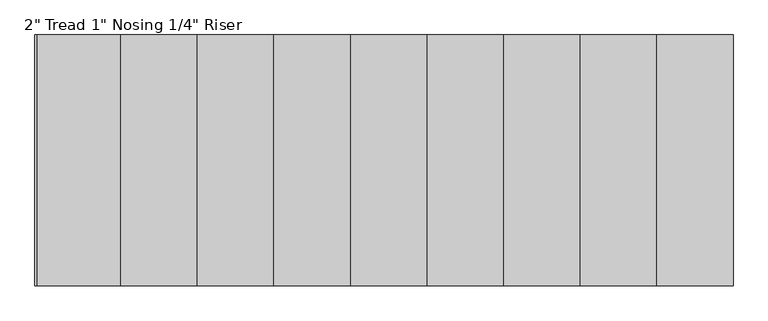
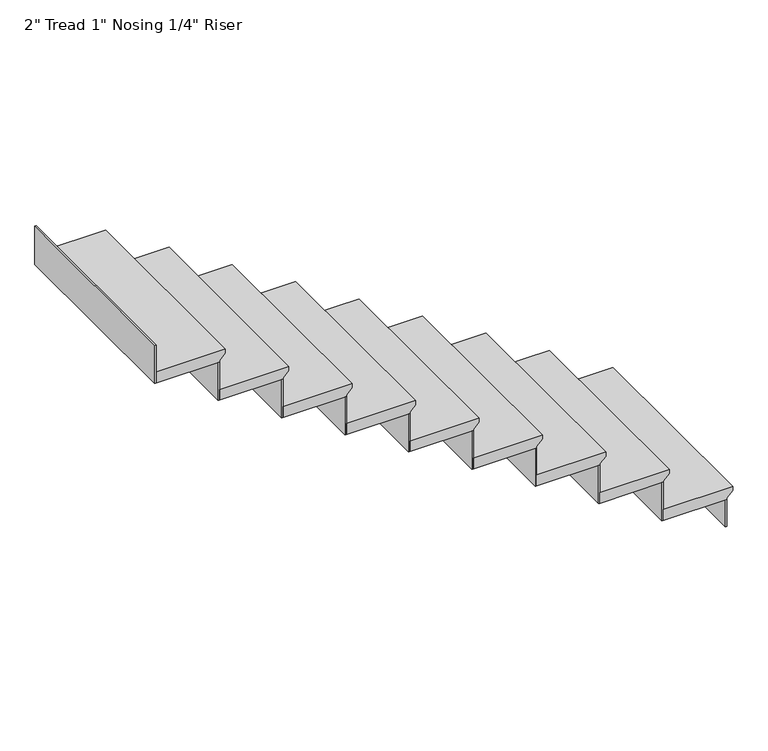
"""IFC4 building model written with IfcOpenShell, lengths in millimetres: stair flight geometry."""

from ifc_helpers import new_model, si_unit, origin, place, context, project, spatial, faceted_brep, source, transform, mapped, element, save


def stair_flight_7bdf39d0(model_context):
    return source(origin(), model_context, "Body", "Brep", [
        faceted_brep([(-9543.8120641, -2647.9669819, 768.35), (-9543.8120641, -2647.9669819, 787.4), (-9543.8120641, -3562.3669819, 787.4), (-9543.8120641, -3562.3669819, 768.35), (-9569.2120641, -2647.9669819, 742.95), (-9569.2120641, -3562.3669819, 742.95), (-9848.6120641, -2647.9669819, 787.4), (-9848.6120641, -3562.3669819, 787.4), (-9569.2120641, -3562.3669819, 736.6), (-9848.6120641, -3562.3669819, 736.6), (-9848.6120641, -2647.9669819, 736.6), (-9569.2120641, -2647.9669819, 736.6)], [[[0, 1, 2, 3]], [[4, 0, 3, 5]], [[2, 1, 6, 7]], [[8, 9, 10, 11]], [[2, 7, 9, 8, 5, 3]], [[8, 11, 4, 5]], [[6, 1, 0, 4, 11, 10]], [[7, 6, 10, 9]]]),
        faceted_brep([(-9569.2120641, -2647.9669819, 736.6), (-9569.2120641, -2647.9669819, 609.6), (-9575.5620641, -2647.9669819, 609.6), (-9575.5620641, -2647.9669819, 736.6), (-9569.2120641, -3562.3669819, 736.6), (-9575.5620641, -3562.3669819, 736.6), (-9575.5620641, -3562.3669819, 609.6), (-9569.2120641, -3562.3669819, 609.6)], [[[0, 1, 2, 3]], [[4, 5, 6, 7]], [[1, 0, 4, 7]], [[2, 1, 7, 6]], [[3, 2, 6, 5]], [[0, 3, 5, 4]]]),
        faceted_brep([(-9848.6120641, -2647.9669819, 914.4), (-9848.6120641, -2647.9669819, 736.6), (-9854.9620641, -2647.9669819, 736.6), (-9854.9620641, -2647.9669819, 914.4), (-9848.6120641, -3562.3669819, 914.4), (-9854.9620641, -3562.3669819, 914.4), (-9854.9620641, -3562.3669819, 736.6), (-9848.6120641, -3562.3669819, 736.6)], [[[0, 1, 2, 3]], [[4, 5, 6, 7]], [[1, 0, 4, 7]], [[2, 1, 7, 6]], [[3, 2, 6, 5]], [[0, 3, 5, 4]]]),
        faceted_brep([(-9823.2120641, -3562.3669819, 965.2), (-9823.2120641, -2647.9669819, 965.2), (-10128.0120641, -2647.9669819, 965.2), (-10128.0120641, -3562.3669819, 965.2), (-9848.6120641, -3562.3669819, 914.4), (-10128.0120641, -3562.3669819, 914.4), (-10128.0120641, -2647.9669819, 914.4), (-9848.6120641, -2647.9669819, 914.4), (-9848.6120641, -3562.3669819, 920.75), (-9823.2120641, -3562.3669819, 946.15), (-9848.6120641, -2647.9669819, 920.75), (-9823.2120641, -2647.9669819, 946.15)], [[[0, 1, 2, 3]], [[4, 5, 6, 7]], [[0, 3, 5, 4, 8, 9]], [[4, 7, 10, 8]], [[2, 1, 11, 10, 7, 6]], [[3, 2, 6, 5]], [[11, 1, 0, 9]], [[10, 11, 9, 8]]]),
        faceted_brep([(-10128.0120641, -2647.9669819, 1092.2), (-10128.0120641, -2647.9669819, 914.4), (-10134.3620641, -2647.9669819, 914.4), (-10134.3620641, -2647.9669819, 1092.2), (-10128.0120641, -3562.3669819, 1092.2), (-10134.3620641, -3562.3669819, 1092.2), (-10134.3620641, -3562.3669819, 914.4), (-10128.0120641, -3562.3669819, 914.4)], [[[0, 1, 2, 3]], [[4, 5, 6, 7]], [[1, 0, 4, 7]], [[2, 1, 7, 6]], [[3, 2, 6, 5]], [[0, 3, 5, 4]]]),
        faceted_brep([(-10102.6120641, -3562.3669819, 1143.0), (-10102.6120641, -2647.9669819, 1143.0), (-10407.4120641, -2647.9669819, 1143.0), (-10407.4120641, -3562.3669819, 1143.0), (-10128.0120641, -3562.3669819, 1092.2), (-10407.4120641, -3562.3669819, 1092.2), (-10407.4120641, -2647.9669819, 1092.2), (-10128.0120641, -2647.9669819, 1092.2), (-10128.0120641, -3562.3669819, 1098.55), (-10102.6120641, -3562.3669819, 1123.95), (-10128.0120641, -2647.9669819, 1098.55), (-10102.6120641, -2647.9669819, 1123.95)], [[[0, 1, 2, 3]], [[4, 5, 6, 7]], [[0, 3, 5, 4, 8, 9]], [[4, 7, 10, 8]], [[2, 1, 11, 10, 7, 6]], [[3, 2, 6, 5]], [[11, 1, 0, 9]], [[10, 11, 9, 8]]]),
        faceted_brep([(-10407.4120641, -2647.9669819, 1270.0), (-10407.4120641, -2647.9669819, 1092.2), (-10413.7620641, -2647.9669819, 1092.2), (-10413.7620641, -2647.9669819, 1270.0), (-10407.4120641, -3562.3669819, 1270.0), (-10413.7620641, -3562.3669819, 1270.0), (-10413.7620641, -3562.3669819, 1092.2), (-10407.4120641, -3562.3669819, 1092.2)], [[[0, 1, 2, 3]], [[4, 5, 6, 7]], [[1, 0, 4, 7]], [[2, 1, 7, 6]], [[3, 2, 6, 5]], [[0, 3, 5, 4]]]),
        faceted_brep([(-10382.0120641, -3562.3669819, 1320.8), (-10382.0120641, -2647.9669819, 1320.8), (-10686.8120641, -2647.9669819, 1320.8), (-10686.8120641, -3562.3669819, 1320.8), (-10407.4120641, -3562.3669819, 1270.0), (-10686.8120641, -3562.3669819, 1270.0), (-10686.8120641, -2647.9669819, 1270.0), (-10407.4120641, -2647.9669819, 1270.0), (-10407.4120641, -3562.3669819, 1276.35), (-10382.0120641, -3562.3669819, 1301.75), (-10407.4120641, -2647.9669819, 1276.35), (-10382.0120641, -2647.9669819, 1301.75)], [[[0, 1, 2, 3]], [[4, 5, 6, 7]], [[0, 3, 5, 4, 8, 9]], [[4, 7, 10, 8]], [[2, 1, 11, 10, 7, 6]], [[3, 2, 6, 5]], [[11, 1, 0, 9]], [[10, 11, 9, 8]]]),
        faceted_brep([(-10686.8120641, -2647.9669819, 1447.8), (-10686.8120641, -2647.9669819, 1270.0), (-10693.1620641, -2647.9669819, 1270.0), (-10693.1620641, -2647.9669819, 1447.8), (-10686.8120641, -3562.3669819, 1447.8), (-10693.1620641, -3562.3669819, 1447.8), (-10693.1620641, -3562.3669819, 1270.0), (-10686.8120641, -3562.3669819, 1270.0)], [[[0, 1, 2, 3]], [[4, 5, 6, 7]], [[1, 0, 4, 7]], [[2, 1, 7, 6]], [[3, 2, 6, 5]], [[0, 3, 5, 4]]]),
        faceted_brep([(-10661.4120641, -3562.3669819, 1498.6), (-10661.4120641, -2647.9669819, 1498.6), (-10966.2120641, -2647.9669819, 1498.6), (-10966.2120641, -3562.3669819, 1498.6), (-10686.8120641, -3562.3669819, 1447.8), (-10966.2120641, -3562.3669819, 1447.8), (-10966.2120641, -2647.9669819, 1447.8), (-10686.8120641, -2647.9669819, 1447.8), (-10686.8120641, -3562.3669819, 1454.15), (-10661.4120641, -3562.3669819, 1479.55), (-10686.8120641, -2647.9669819, 1454.15), (-10661.4120641, -2647.9669819, 1479.55)], [[[0, 1, 2, 3]], [[4, 5, 6, 7]], [[0, 3, 5, 4, 8, 9]], [[4, 7, 10, 8]], [[2, 1, 11, 10, 7, 6]], [[3, 2, 6, 5]], [[11, 1, 0, 9]], [[10, 11, 9, 8]]]),
        faceted_brep([(-10966.2120641, -2647.9669819, 1625.6), (-10966.2120641, -2647.9669819, 1447.8), (-10972.5620641, -2647.9669819, 1447.8), (-10972.5620641, -2647.9669819, 1625.6), (-10966.2120641, -3562.3669819, 1625.6), (-10972.5620641, -3562.3669819, 1625.6), (-10972.5620641, -3562.3669819, 1447.8), (-10966.2120641, -3562.3669819, 1447.8)], [[[0, 1, 2, 3]], [[4, 5, 6, 7]], [[1, 0, 4, 7]], [[2, 1, 7, 6]], [[3, 2, 6, 5]], [[0, 3, 5, 4]]]),
        faceted_brep([(-10940.8120641, -3562.3669819, 1676.4), (-10940.8120641, -2647.9669819, 1676.4), (-11245.6120641, -2647.9669819, 1676.4), (-11245.6120641, -3562.3669819, 1676.4), (-10966.2120641, -3562.3669819, 1625.6), (-11245.6120641, -3562.3669819, 1625.6), (-11245.6120641, -2647.9669819, 1625.6), (-10966.2120641, -2647.9669819, 1625.6), (-10966.2120641, -3562.3669819, 1631.95), (-10940.8120641, -3562.3669819, 1657.35), (-10966.2120641, -2647.9669819, 1631.95), (-10940.8120641, -2647.9669819, 1657.35)], [[[0, 1, 2, 3]], [[4, 5, 6, 7]], [[0, 3, 5, 4, 8, 9]], [[4, 7, 10, 8]], [[2, 1, 11, 10, 7, 6]], [[3, 2, 6, 5]], [[11, 1, 0, 9]], [[10, 11, 9, 8]]]),
        faceted_brep([(-11245.6120641, -2647.9669819, 1803.4), (-11245.6120641, -2647.9669819, 1625.6), (-11251.9620641, -2647.9669819, 1625.6), (-11251.9620641, -2647.9669819, 1803.4), (-11245.6120641, -3562.3669819, 1803.4), (-11251.9620641, -3562.3669819, 1803.4), (-11251.9620641, -3562.3669819, 1625.6), (-11245.6120641, -3562.3669819, 1625.6)], [[[0, 1, 2, 3]], [[4, 5, 6, 7]], [[1, 0, 4, 7]], [[2, 1, 7, 6]], [[3, 2, 6, 5]], [[0, 3, 5, 4]]]),
        faceted_brep([(-11220.2120641, -3562.3669819, 1854.2), (-11220.2120641, -2647.9669819, 1854.2), (-11525.0120641, -2647.9669819, 1854.2), (-11525.0120641, -3562.3669819, 1854.2), (-11245.6120641, -3562.3669819, 1803.4), (-11525.0120641, -3562.3669819, 1803.4), (-11525.0120641, -2647.9669819, 1803.4), (-11245.6120641, -2647.9669819, 1803.4), (-11245.6120641, -3562.3669819, 1809.75), (-11220.2120641, -3562.3669819, 1835.15), (-11245.6120641, -2647.9669819, 1809.75), (-11220.2120641, -2647.9669819, 1835.15)], [[[0, 1, 2, 3]], [[4, 5, 6, 7]], [[0, 3, 5, 4, 8, 9]], [[4, 7, 10, 8]], [[2, 1, 11, 10, 7, 6]], [[3, 2, 6, 5]], [[11, 1, 0, 9]], [[10, 11, 9, 8]]]),
        faceted_brep([(-11525.0120641, -2647.9669819, 1981.2), (-11525.0120641, -2647.9669819, 1803.4), (-11531.3620641, -2647.9669819, 1803.4), (-11531.3620641, -2647.9669819, 1981.2), (-11525.0120641, -3562.3669819, 1981.2), (-11531.3620641, -3562.3669819, 1981.2), (-11531.3620641, -3562.3669819, 1803.4), (-11525.0120641, -3562.3669819, 1803.4)], [[[0, 1, 2, 3]], [[4, 5, 6, 7]], [[1, 0, 4, 7]], [[2, 1, 7, 6]], [[3, 2, 6, 5]], [[0, 3, 5, 4]]]),
        faceted_brep([(-11499.6120641, -3562.3669819, 2032.0), (-11499.6120641, -2647.9669819, 2032.0), (-11804.4120641, -2647.9669819, 2032.0), (-11804.4120641, -3562.3669819, 2032.0), (-11525.0120641, -3562.3669819, 1981.2), (-11804.4120641, -3562.3669819, 1981.2), (-11804.4120641, -2647.9669819, 1981.2), (-11525.0120641, -2647.9669819, 1981.2), (-11525.0120641, -3562.3669819, 1987.55), (-11499.6120641, -3562.3669819, 2012.95), (-11525.0120641, -2647.9669819, 1987.55), (-11499.6120641, -2647.9669819, 2012.95)], [[[0, 1, 2, 3]], [[4, 5, 6, 7]], [[0, 3, 5, 4, 8, 9]], [[4, 7, 10, 8]], [[2, 1, 11, 10, 7, 6]], [[3, 2, 6, 5]], [[11, 1, 0, 9]], [[10, 11, 9, 8]]]),
        faceted_brep([(-12083.8120641, -2647.9669819, 2336.8), (-12083.8120641, -2647.9669819, 2159.0), (-12090.1620641, -2647.9669819, 2159.0), (-12090.1620641, -2647.9669819, 2336.8), (-12083.8120641, -3562.3669819, 2336.8), (-12090.1620641, -3562.3669819, 2336.8), (-12090.1620641, -3562.3669819, 2159.0), (-12083.8120641, -3562.3669819, 2159.0)], [[[0, 1, 2, 3]], [[4, 5, 6, 7]], [[1, 0, 4, 7]], [[2, 1, 7, 6]], [[3, 2, 6, 5]], [[0, 3, 5, 4]]]),
        faceted_brep([(-11804.4120641, -2647.9669819, 2159.0), (-11804.4120641, -2647.9669819, 1981.2), (-11810.7620641, -2647.9669819, 1981.2), (-11810.7620641, -2647.9669819, 2159.0), (-11804.4120641, -3562.3669819, 2159.0), (-11810.7620641, -3562.3669819, 2159.0), (-11810.7620641, -3562.3669819, 1981.2), (-11804.4120641, -3562.3669819, 1981.2)], [[[0, 1, 2, 3]], [[4, 5, 6, 7]], [[1, 0, 4, 7]], [[2, 1, 7, 6]], [[3, 2, 6, 5]], [[0, 3, 5, 4]]]),
        faceted_brep([(-11779.0120641, -3562.3669819, 2209.8), (-11779.0120641, -2647.9669819, 2209.8), (-12058.4120641, -2647.9669819, 2209.8), (-12083.8120641, -2647.9669819, 2209.8), (-12083.8120641, -3562.3669819, 2209.8), (-11804.4120641, -3562.3669819, 2159.0), (-12083.8120641, -3562.3669819, 2159.0), (-12083.8120641, -2647.9669819, 2159.0), (-12058.4120641, -2647.9669819, 2159.0), (-11804.4120641, -2647.9669819, 2159.0), (-11804.4120641, -3562.3669819, 2165.35), (-11779.0120641, -3562.3669819, 2190.75), (-11804.4120641, -2647.9669819, 2165.35), (-11779.0120641, -2647.9669819, 2190.75)], [[[0, 1, 2, 3, 4]], [[5, 6, 7, 8, 9]], [[0, 4, 6, 5, 10, 11]], [[5, 9, 12, 10]], [[2, 1, 13, 12, 9, 8]], [[3, 2, 8, 7]], [[4, 3, 7, 6]], [[13, 1, 0, 11]], [[12, 13, 11, 10]]]),
    ])


if __name__ == "__main__":
    model = new_model("IFC4")
    model_context = context("Model", 3, world=origin())
    ifc_project = project(units=[si_unit("LENGTHUNIT", "METRE", prefix="MILLI")], contexts=[model_context])
    site = spatial("IfcSite", under=ifc_project)
    building = spatial("IfcBuilding", under=site)
    placement = place(None, origin())
    stair_flight_shape = stair_flight_7bdf39d0(model_context)
    element("IfcStairFlight", 1, ObjectType="2\" Tread 1\" Nosing 1/4\" Riser", at=placement, inside=building, context=model_context, shape_type="MappedRepresentation", body=[
        mapped(stair_flight_shape, transform((0.0, 0.0, 0.0), x_axis=(1.0, 0.0, 0.0), y_axis=(0.0, 1.0, 0.0), z_axis=(0.0, 0.0, 1.0))),
    ])
    save(model, "model.ifc")
